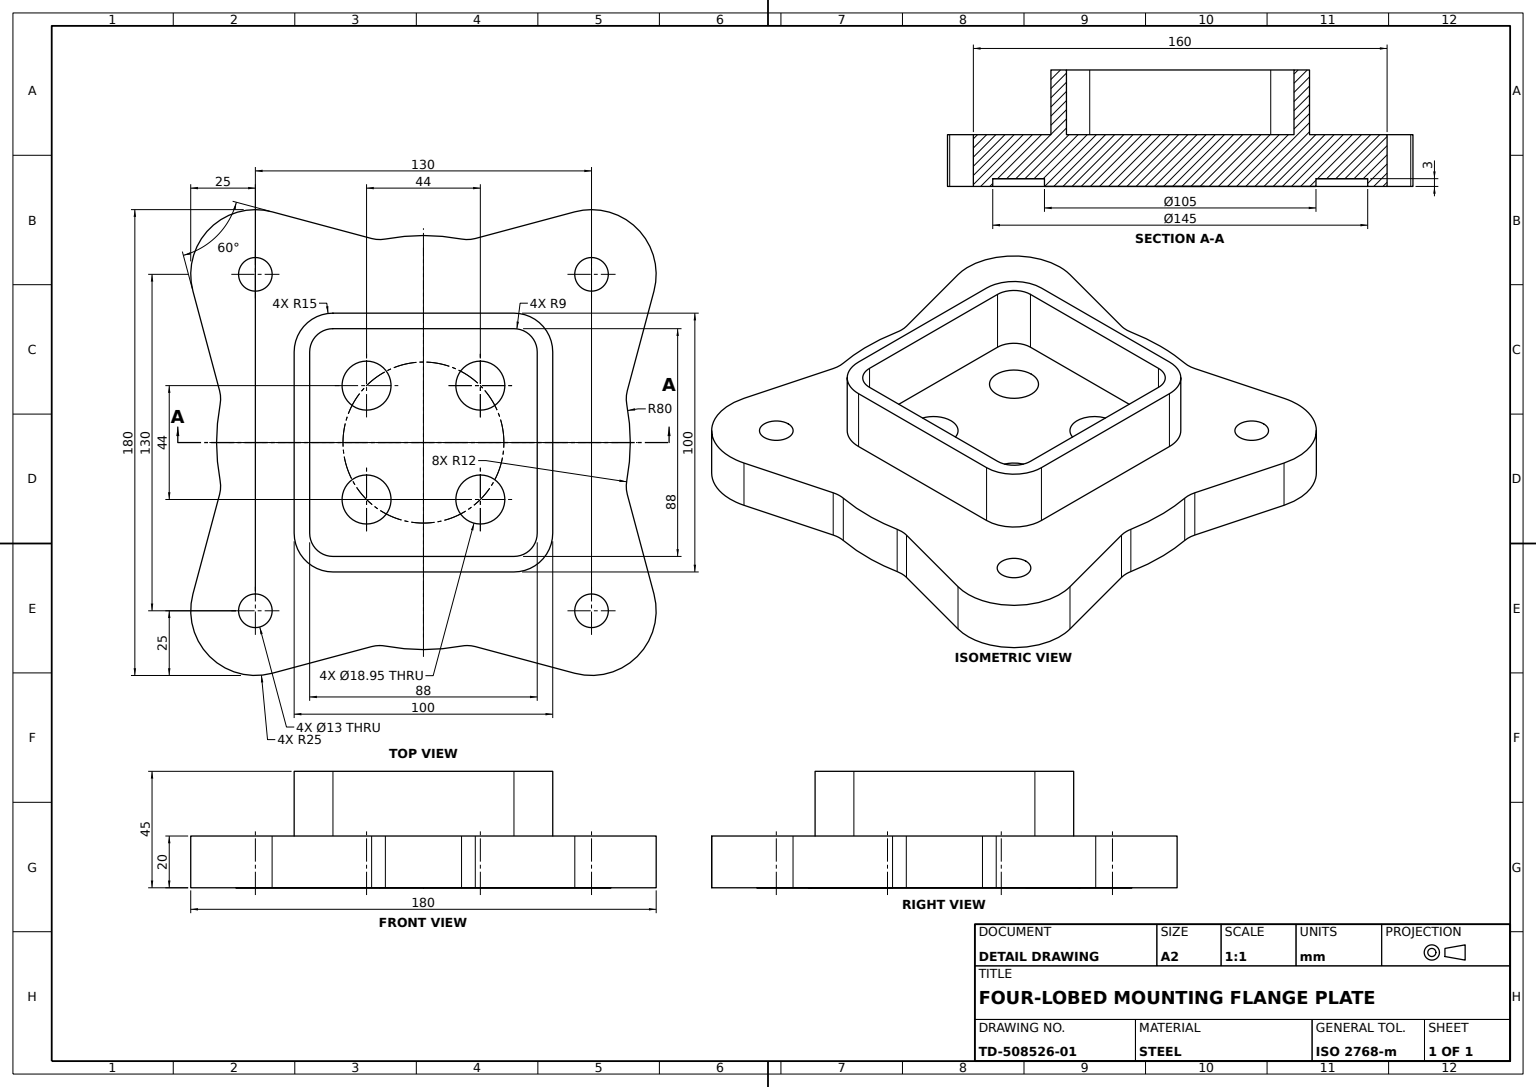
from build123d import *

# Parameters (mm, degrees)
BASE_FLANGE_SKETCH_R      = 6.5
BASE_FLANGE_DEPTH         = 10
SQUARE_BOSS_DEPTH         = 25
BOSS_POCKET_DEPTH         = 130.711217711
BOSS_POCKET_DEPTH_BACK    = 130.711217711
BOSS_POCKET_SKETCH_R      = 9.473120825
RECESS_CUT_3MM_DEPTH      = 136
RECESS_CUT_3MM_DEPTH_BACK = 3
RECESS_SKETCH_R           = 72.5
RECESS_SKETCH_R_2         = 52.5


with BuildPart() as part:
    # Base Flange Sketch → Base Flange (new, symmetric)
    with BuildSketch(Plane(origin=(0, 0, 0), x_dir=(1, 0, 0), z_dir=(0, 1, 0))):
        with BuildLine():
            Line((-89.148145657, 58.529523872), (-78.836109635, 20.044481509))
            ThreePointArc((-78.836109635, 20.044481509), (-78.436026062, 17.398303615), (-78.632364827, 14.72926345))
            ThreePointArc((-78.632364827, 14.72926345), (-80, 0), (-78.632364827, -14.72926345))
            ThreePointArc((-78.632364827, -14.72926345), (-78.436026062, -17.398303615), (-78.836109635, -20.044481509))
            Line((-78.836109635, -20.044481509), (-89.148145657, -58.529523872))
            ThreePointArc((-89.148145657, -58.529523872), (-82.67766953, -82.67766953), (-58.529523872, -89.148145657))
            Line((-58.529523872, -89.148145657), (-20.044481509, -78.836109635))
            ThreePointArc((-20.044481509, -78.836109635), (-17.398303615, -78.436026062), (-14.72926345, -78.632364827))
            ThreePointArc((-14.72926345, -78.632364827), (0, -80), (14.72926345, -78.632364827))
            ThreePointArc((14.72926345, -78.632364827), (17.398303615, -78.436026062), (20.044481509, -78.836109635))
            Line((20.044481509, -78.836109635), (58.529523872, -89.148145657))
            ThreePointArc((58.529523872, -89.148145657), (82.67766953, -82.67766953), (89.148145657, -58.529523872))
            Line((89.148145657, -58.529523872), (78.836109635, -20.044481509))
            ThreePointArc((78.836109635, -20.044481509), (78.436026062, -17.398303615), (78.632364827, -14.72926345))
            ThreePointArc((78.632364827, -14.72926345), (80, 0), (78.632364827, 14.72926345))
            ThreePointArc((78.632364827, 14.72926345), (78.436026062, 17.398303615), (78.836109635, 20.044481509))
            Line((78.836109635, 20.044481509), (89.148145657, 58.529523872))
            ThreePointArc((89.148145657, 58.529523872), (82.67766953, 82.67766953), (58.529523872, 89.148145657))
            Line((58.529523872, 89.148145657), (20.044481509, 78.836109635))
            ThreePointArc((20.044481509, 78.836109635), (17.398303615, 78.436026062), (14.72926345, 78.632364827))
            ThreePointArc((14.72926345, 78.632364827), (0, 80), (-14.72926345, 78.632364827))
            ThreePointArc((-14.72926345, 78.632364827), (-17.398303615, 78.436026062), (-20.044481509, 78.836109635))
            Line((-20.044481509, 78.836109635), (-58.529523872, 89.148145657))
            ThreePointArc((-58.529523872, 89.148145657), (-82.67766953, 82.67766953), (-89.148145657, 58.529523872))
        make_face()
        with Locations(Location((-65, 65, 0), (0, 0, 270))):
            Circle(BASE_FLANGE_SKETCH_R, mode=Mode.SUBTRACT)
        with Locations(Location((65, 65, 0), (0, 0, 270))):
            Circle(BASE_FLANGE_SKETCH_R, mode=Mode.SUBTRACT)
        with Locations(Location((65, -65, 0), (0, 0, 270))):
            Circle(BASE_FLANGE_SKETCH_R, mode=Mode.SUBTRACT)
        with Locations(Location((-65, -65, 0), (0, 0, 270))):
            Circle(BASE_FLANGE_SKETCH_R, mode=Mode.SUBTRACT)
    extrude(amount=BASE_FLANGE_DEPTH, both=True)

    # Square Boss Sketch → Square Boss (add)
    with BuildSketch(Plane(origin=(0, 10, 0), x_dir=(1, 0, 0), z_dir=(0, 1, 0))):
        with BuildLine():
            Line((-35, 50), (35, 50))
            ThreePointArc((35, 50), (45.606601718, 45.606601718), (50, 35))
            Line((50, 35), (50, -35))
            ThreePointArc((50, -35), (45.606601718, -45.606601718), (35, -50))
            Line((35, -50), (-35, -50))
            ThreePointArc((-35, -50), (-45.606601718, -45.606601718), (-50, -35))
            Line((-50, -35), (-50, 35))
            ThreePointArc((-50, 35), (-45.606601718, 45.606601718), (-35, 50))
        make_face()
        with BuildLine():
            ThreePointArc((-35, 44), (-41.363961031, 41.363961031), (-44, 35))
            Line((-44, 35), (-44, -35))
            ThreePointArc((-44, -35), (-41.363961031, -41.363961031), (-35, -44))
            Line((-35, -44), (35, -44))
            ThreePointArc((35, -44), (41.363961031, -41.363961031), (44, -35))
            Line((44, -35), (44, 35))
            ThreePointArc((44, 35), (41.363961031, 41.363961031), (35, 44))
            Line((35, 44), (-35, 44))
        make_face(mode=Mode.SUBTRACT)
    extrude(amount=SQUARE_BOSS_DEPTH)

    # Boss Pocket Sketch → Boss Pocket (cut, two sides: drawn at the far end of the back side and taken through both)
    with BuildSketch(Plane(origin=(0, 10, 0), x_dir=(1, 0, 0), z_dir=(0, 1, 0)).offset(-BOSS_POCKET_DEPTH_BACK)):
        with Locations(Location((-22, -22, 0), (0, 0, 270))):
            Circle(BOSS_POCKET_SKETCH_R)
        with Locations(Location((22, -22, 0), (0, 0, 270))):
            Circle(BOSS_POCKET_SKETCH_R)
        with Locations(Location((22, 22, 0), (0, 0, 270))):
            Circle(BOSS_POCKET_SKETCH_R)
        with Locations(Location((-22, 22, 0), (0, 0, 270))):
            Circle(BOSS_POCKET_SKETCH_R)
    extrude(amount=BOSS_POCKET_DEPTH + BOSS_POCKET_DEPTH_BACK, mode=Mode.SUBTRACT)

    # Recess Sketch → Recess Cut 3mm (cut, two sides: drawn at the far end of the back side and taken through both)
    with BuildSketch(Plane.XZ.offset(10).offset(-RECESS_CUT_3MM_DEPTH_BACK)):
        with Locations(Location((0, 0, 0), (0, 0, 270))):
            Circle(RECESS_SKETCH_R)
        with Locations(Location((0, 0, 0), (0, 0, 270))):
            Circle(RECESS_SKETCH_R_2, mode=Mode.SUBTRACT)
    extrude(amount=RECESS_CUT_3MM_DEPTH + RECESS_CUT_3MM_DEPTH_BACK, mode=Mode.SUBTRACT)


solid = part.part
